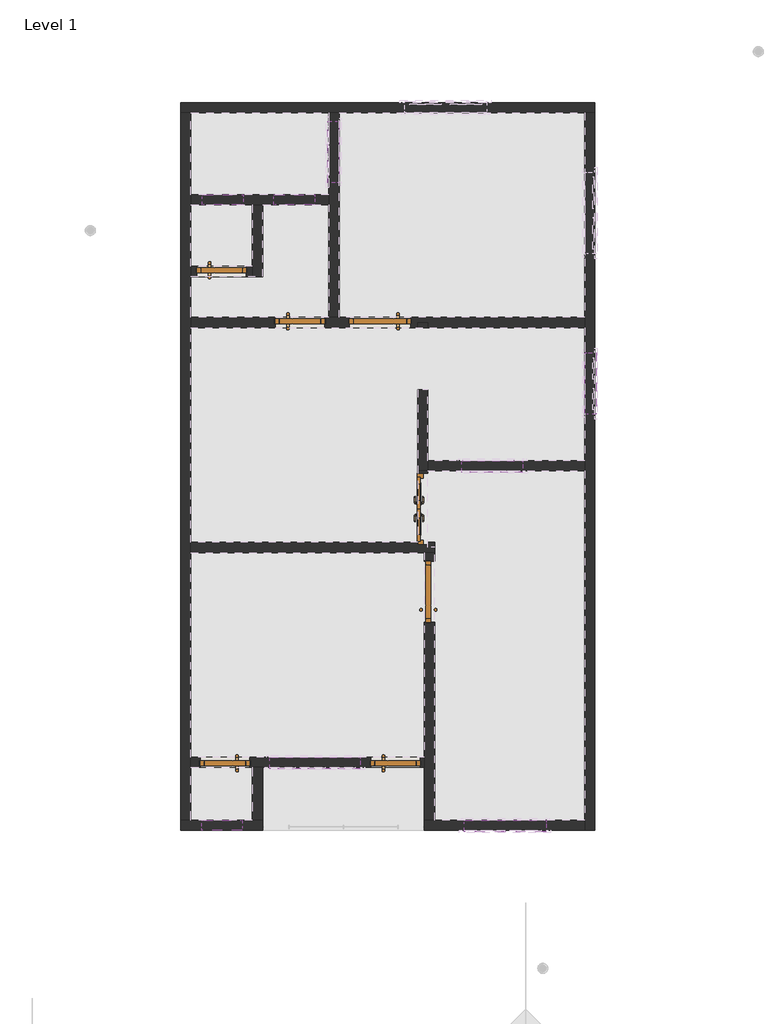
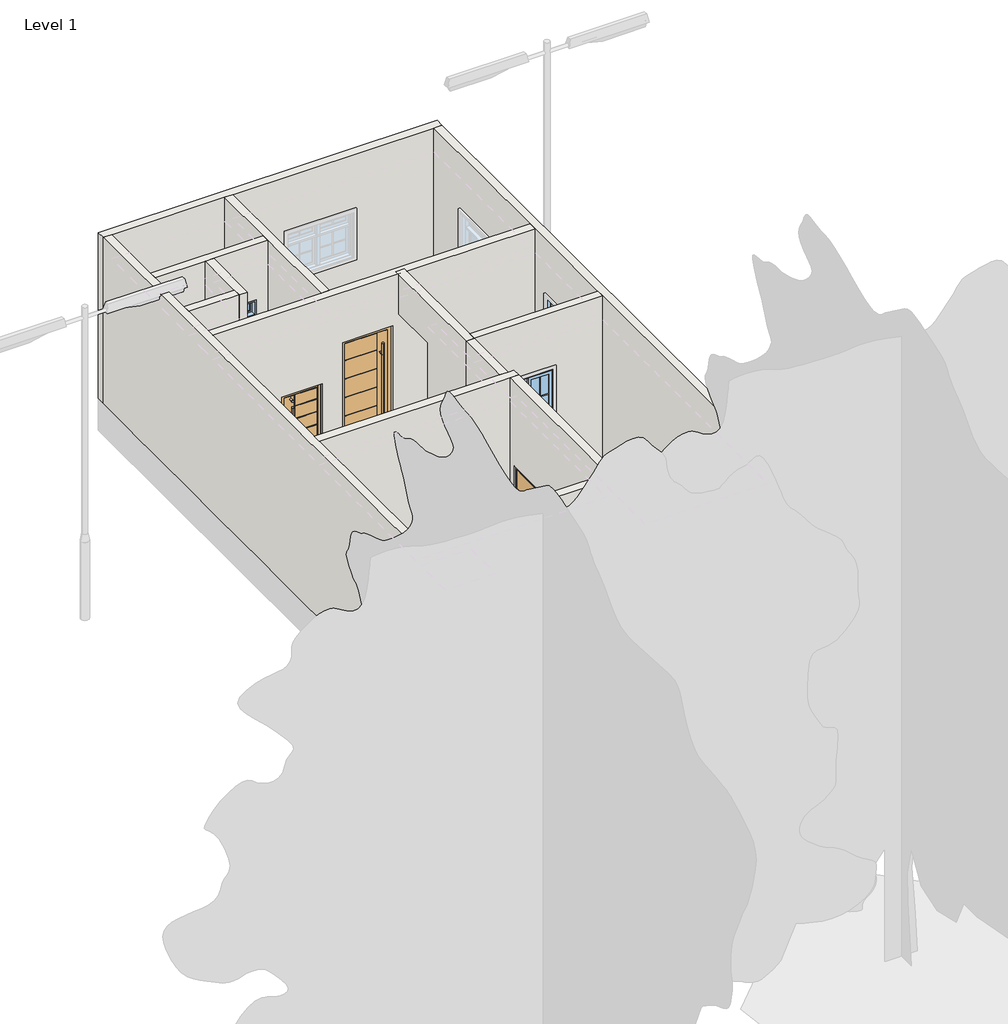
# One storey, part 1 of 2: 17 walls, 8 windows, 7 doors.
"""IFC4 building model written with IfcOpenShell, lengths in millimetres."""

from ifc_helpers import new_model, si_unit, frame, origin, place, context, project, spatial, polyline, outline, extrude, faceted_brep, transform, mapped, element, save
from components import door_9b787682, door_dc81b0c5, door_3_5c4206ef, door_3_79df91aa, door_2576ec39, door_55c03dfd, fixed_2_65c13adb, window_61697a4f, m_window_casement_double_3_e0bd8fa3, m_window_casement_double_awning_double_4_7efa9bbd

model = new_model("IFC4")

# Units and contexts
model_context = context("Model", 3, world=origin())
ifc_project = project(units=[si_unit("LENGTHUNIT", "METRE", prefix="MILLI")], contexts=[model_context])

# Site, building, storey
site = spatial("IfcSite", under=ifc_project)
building = spatial("IfcBuilding", under=site)
storey = spatial("IfcBuildingStorey", under=building, Name="Level 1", Elevation=0.0)

# Doors
placement = place(None, origin())
door_shape = door_9b787682(model_context)
element("IfcDoor", 1, ObjectType="2'5\"", at=placement, inside=storey, context=model_context, shape_type="MappedRepresentation", body=[
    mapped(door_shape, transform((-22033.2963079, 3049.4742053, 655.8445349), x_axis=(1.0, 0.0, 0.0), y_axis=(0.0, 1.0, 0.0), z_axis=(0.0, 0.0, 1.0))),
])
element("IfcDoor", 2, ObjectType="2'5\"", at=placement, inside=storey, context=model_context, shape_type="MappedRepresentation", body=[
    mapped(door_shape, transform((-23201.6963079, 3811.4742053, 655.8445349), x_axis=(1.0, 0.0, 0.0), y_axis=(0.0, 1.0, 0.0), z_axis=(0.0, 0.0, 1.0))),
])
element("IfcDoor", 3, ObjectType="2'5\"", at=placement, inside=storey, context=model_context, shape_type="MappedRepresentation", body=[
    mapped(door_shape, transform((-23150.8963079, -3503.7257947, 655.8445349), x_axis=(-1.0, 0.0, 0.0), y_axis=(0.0, -1.0, 0.0), z_axis=(0.0, 0.0, 1.0))),
])
door_2_shape = door_dc81b0c5(model_context)
element("IfcDoor", 4, ObjectType="2'5\"", at=placement, inside=storey, context=model_context, shape_type="MappedRepresentation", body=[
    mapped(door_2_shape, transform((-20610.8963079, -3503.7257947, 655.8445349), x_axis=(1.0, 0.0, 0.0), y_axis=(0.0, 1.0, 0.0), z_axis=(0.0, 0.0, 1.0))),
])
door_3_shape = door_3_5c4206ef(model_context)
element("IfcDoor", 5, ObjectType="3'", at=placement, inside=storey, context=model_context, shape_type="MappedRepresentation", body=[
    mapped(door_3_shape, transform((-20102.8963079, -963.7257947, 0.0), x_axis=(0.0, 1.0, 0.0), y_axis=(-1.0, 0.0, 0.0), z_axis=(0.0, 0.0, 1.0))),
])
door_3_2_shape = door_3_79df91aa(model_context)
element("IfcDoor", 6, ObjectType="3'", at=placement, inside=storey, context=model_context, shape_type="MappedRepresentation", body=[
    mapped(door_3_2_shape, transform((-20839.4963079, 3049.4742053, 655.8445349), x_axis=(-1.0, 0.0, 0.0), y_axis=(0.0, -1.0, 0.0), z_axis=(0.0, 0.0, 1.0))),
])
door_4_shape = door_2576ec39(model_context)
door_5_shape = door_55c03dfd(model_context)
element("IfcDoor", 7, ObjectType="ExtDbl (8) : 3'6\"", at=placement, inside=storey, context=model_context, shape_type="MappedRepresentation", body=[
    mapped(door_4_shape, transform((-20204.4963079, 268.1742053, 0.0), x_axis=(0.0, -1.0, 0.0), y_axis=(1.0, 0.0, 0.0), z_axis=(0.0, 0.0, 1.0))),
    mapped(door_5_shape, transform((-20204.4963079, 268.1742053, 0.0), x_axis=(0.0, -1.0, 0.0), y_axis=(1.0, 0.0, 0.0), z_axis=(0.0, 0.0, 1.0))),
])

# Walls
element("IfcWall", 8, ObjectType="Generic - 6\"", at=placement, inside=storey, context=model_context, shape_type="Brep", body=[
    faceted_brep([(-23811.2963079, 6173.6742053, 609.6), (-23658.8963079, 6173.6742053, 609.6), (-21601.4963079, 6173.6742053, 609.6), (-21449.0963079, 6173.6742053, 609.6), (-17791.4963079, 6173.6742053, 609.6), (-17639.0963079, 6173.6742053, 609.6), (-17639.0963079, 6173.6742053, 3810.0), (-17791.4963079, 6173.6742053, 3810.0), (-21449.0963079, 6173.6742053, 3810.0), (-21601.4963079, 6173.6742053, 3810.0), (-23658.8963079, 6173.6742053, 3810.0), (-23811.2963079, 6173.6742053, 3810.0), (-19251.9963079, 6173.6742053, 2728.8), (-19251.9963079, 6173.6742053, 1828.8), (-20471.1963079, 6173.6742053, 1828.8), (-20471.1963079, 6173.6742053, 2728.8), (-23811.2963079, 6326.0742053, 609.6), (-23811.2963079, 6326.0742053, 3810.0), (-17639.0963079, 6326.0742053, 3810.0), (-17639.0963079, 6326.0742053, 609.6), (-19251.9963079, 6326.0742053, 2728.8), (-20471.1963079, 6326.0742053, 2728.8), (-20471.1963079, 6326.0742053, 1828.8), (-19251.9963079, 6326.0742053, 1828.8)], [[[0, 1, 2, 3, 4, 5, 6, 7, 8, 9, 10, 11], [12, 13, 14, 15]], [[16, 17, 18, 19], [20, 21, 22, 23]], [[5, 4, 3, 2, 1, 0, 16, 19]], [[11, 10, 9, 8, 7, 6, 18, 17]], [[6, 5, 19, 18]], [[0, 11, 17, 16]], [[13, 12, 20, 23]], [[14, 13, 23, 22]], [[15, 14, 22, 21]], [[12, 15, 21, 20]]]),
])
element("IfcWall", 9, ObjectType="Generic - 6\"", at=placement, inside=storey, context=model_context, shape_type="Brep", body=[
    faceted_brep([(-17791.4963079, 6173.6742053, 609.6), (-17791.4963079, 3125.6742053, 609.6), (-17791.4963079, 2973.2742053, 609.6), (-17791.4963079, 992.0742053, 609.6), (-17791.4963079, 839.6742053, 609.6), (-17791.4963079, -4367.3257947, 609.6), (-17791.4963079, -4519.7257947, 609.6), (-17791.4963079, -4519.7257947, 3810.0), (-17791.4963079, -4367.3257947, 3810.0), (-17791.4963079, 839.6742053, 3810.0), (-17791.4963079, 992.0742053, 3810.0), (-17791.4963079, 2973.2742053, 3810.0), (-17791.4963079, 3125.6742053, 3810.0), (-17791.4963079, 6173.6742053, 3810.0), (-17791.4963079, 4071.8242053, 2728.8), (-17791.4963079, 4071.8242053, 1828.8), (-17791.4963079, 5291.0242053, 1828.8), (-17791.4963079, 5291.0242053, 2728.8), (-17791.4963079, 1682.6367053, 2728.8), (-17791.4963079, 1682.6367053, 1828.8), (-17791.4963079, 2597.0367053, 1828.8), (-17791.4963079, 2597.0367053, 2728.8), (-17639.0963079, 6173.6742053, 609.6), (-17639.0963079, 6173.6742053, 3810.0), (-17639.0963079, -4519.7257947, 3810.0), (-17639.0963079, -4519.7257947, 609.6), (-17639.0963079, 4071.8242053, 2728.8), (-17639.0963079, 5291.0242053, 2728.8), (-17639.0963079, 5291.0242053, 1828.8), (-17639.0963079, 4071.8242053, 1828.8), (-17639.0963079, 1682.6367053, 2728.8), (-17639.0963079, 2597.0367053, 2728.8), (-17639.0963079, 2597.0367053, 1828.8), (-17639.0963079, 1682.6367053, 1828.8)], [[[0, 1, 2, 3, 4, 5, 6, 7, 8, 9, 10, 11, 12, 13], [14, 15, 16, 17], [18, 19, 20, 21]], [[22, 23, 24, 25], [26, 27, 28, 29], [30, 31, 32, 33]], [[6, 5, 4, 3, 2, 1, 0, 22, 25]], [[13, 12, 11, 10, 9, 8, 7, 24, 23]], [[0, 13, 23, 22]], [[7, 6, 25, 24]], [[15, 14, 26, 29]], [[16, 15, 29, 28]], [[17, 16, 28, 27]], [[14, 17, 27, 26]], [[19, 18, 30, 33]], [[20, 19, 33, 32]], [[21, 20, 32, 31]], [[18, 21, 31, 30]]]),
])
element("IfcWall", 10, ObjectType="Generic - 6\"", at=placement, inside=storey, context=model_context, shape_type="Brep", body=[
    faceted_brep([(-17791.4963079, -4367.3257947, 609.6), (-20026.6963079, -4367.3257947, 609.6), (-20179.0963079, -4367.3257947, 609.6), (-20179.0963079, -4367.3257947, 3810.0), (-20026.6963079, -4367.3257947, 3810.0), (-17791.4963079, -4367.3257947, 3810.0), (-19585.5697454, -4367.3257947, 2728.8), (-19585.5697454, -4367.3257947, 1828.8), (-18366.3697454, -4367.3257947, 1828.8), (-18366.3697454, -4367.3257947, 2728.8), (-17791.4963079, -4519.7257947, 609.6), (-17791.4963079, -4519.7257947, 3810.0), (-20179.0963079, -4519.7257947, 3810.0), (-20179.0963079, -4519.7257947, 609.6), (-19585.5697454, -4519.7257947, 2728.8), (-18366.3697454, -4519.7257947, 2728.8), (-18366.3697454, -4519.7257947, 1828.8), (-19585.5697454, -4519.7257947, 1828.8)], [[[0, 1, 2, 3, 4, 5], [6, 7, 8, 9]], [[10, 11, 12, 13], [14, 15, 16, 17]], [[2, 1, 0, 10, 13]], [[5, 4, 3, 12, 11]], [[0, 5, 11, 10]], [[3, 2, 13, 12]], [[7, 6, 14, 17]], [[8, 7, 17, 16]], [[9, 8, 16, 15]], [[6, 9, 15, 14]]]),
])
element("IfcWall", 11, ObjectType="Generic - 6\"", at=placement, inside=storey, context=model_context, shape_type="Brep", body=[
    faceted_brep([(-23811.2963079, -4519.7257947, 609.6), (-22592.0963079, -4519.7257947, 609.6), (-22592.0963079, -4519.7257947, 3810.0), (-23811.2963079, -4519.7257947, 3810.0), (-23500.5431829, -4519.7257947, 2743.2), (-22890.9431829, -4519.7257947, 2743.2), (-22890.9431829, -4519.7257947, 2438.4), (-23500.5431829, -4519.7257947, 2438.4), (-23811.2963079, -4367.3257947, 609.6), (-23811.2963079, -4367.3257947, 3810.0), (-23658.8963079, -4367.3257947, 3810.0), (-22744.4963079, -4367.3257947, 3810.0), (-22592.0963079, -4367.3257947, 3810.0), (-22592.0963079, -4367.3257947, 609.6), (-22744.4963079, -4367.3257947, 609.6), (-23658.8963079, -4367.3257947, 609.6), (-23500.5431829, -4367.3257947, 2743.2), (-23500.5431829, -4367.3257947, 2438.4), (-22890.9431829, -4367.3257947, 2438.4), (-22890.9431829, -4367.3257947, 2743.2)], [[[0, 1, 2, 3], [4, 5, 6, 7]], [[8, 9, 10, 11, 12, 13, 14, 15], [16, 17, 18, 19]], [[1, 0, 8, 15, 14, 13]], [[3, 2, 12, 11, 10, 9]], [[0, 3, 9, 8]], [[2, 1, 13, 12]], [[17, 16, 4, 7]], [[18, 17, 7, 6]], [[19, 18, 6, 5]], [[16, 19, 5, 4]]]),
])
element("IfcWall", 12, ObjectType="Generic - 6\"", at=placement, inside=storey, context=model_context, shape_type="Brep", body=[
    faceted_brep([(-23658.8963079, -4367.3257947, 609.6), (-23658.8963079, -3579.9257947, 609.6), (-23658.8963079, -3427.5257947, 609.6), (-23658.8963079, -379.5257947, 609.6), (-23658.8963079, -227.1257947, 609.6), (-23658.8963079, 2973.2742053, 609.6), (-23658.8963079, 3125.6742053, 609.6), (-23658.8963079, 3735.2742053, 609.6), (-23658.8963079, 3887.6742053, 609.6), (-23658.8963079, 4802.0742053, 609.6), (-23658.8963079, 4954.4742053, 609.6), (-23658.8963079, 6173.6742053, 609.6), (-23658.8963079, 6173.6742053, 3810.0), (-23658.8963079, 4954.4742053, 3810.0), (-23658.8963079, 4802.0742053, 3810.0), (-23658.8963079, 3887.6742053, 3810.0), (-23658.8963079, 3735.2742053, 3810.0), (-23658.8963079, 3125.6742053, 3810.0), (-23658.8963079, 2973.2742053, 3810.0), (-23658.8963079, -227.1257947, 3810.0), (-23658.8963079, -379.5257947, 3810.0), (-23658.8963079, -3427.5257947, 3810.0), (-23658.8963079, -3579.9257947, 3810.0), (-23658.8963079, -4367.3257947, 3810.0), (-23811.2963079, -4367.3257947, 609.6), (-23811.2963079, -4367.3257947, 3810.0), (-23811.2963079, 6173.6742053, 3810.0), (-23811.2963079, 6173.6742053, 609.6)], [[[0, 1, 2, 3, 4, 5, 6, 7, 8, 9, 10, 11, 12, 13, 14, 15, 16, 17, 18, 19, 20, 21, 22, 23]], [[24, 25, 26, 27]], [[11, 10, 9, 8, 7, 6, 5, 4, 3, 2, 1, 0, 24, 27]], [[23, 22, 21, 20, 19, 18, 17, 16, 15, 14, 13, 12, 26, 25]], [[12, 11, 27, 26]], [[0, 23, 25, 24]]]),
])
element("IfcWall", 13, ObjectType="Generic - 6\"", at=placement, inside=storey, context=model_context, shape_type="Brep", body=[
    faceted_brep([(-21601.4963079, 6173.6742053, 609.6), (-21601.4963079, 4954.4742053, 609.6), (-21601.4963079, 4802.0742053, 609.6), (-21601.4963079, 3125.6742053, 609.6), (-21601.4963079, 3125.6742053, 3810.0), (-21601.4963079, 4802.0742053, 3810.0), (-21601.4963079, 4954.4742053, 3810.0), (-21601.4963079, 6173.6742053, 3810.0), (-21601.4963079, 6046.6742053, 2728.8), (-21601.4963079, 5132.2742053, 2728.8), (-21601.4963079, 5132.2742053, 1828.8), (-21601.4963079, 6046.6742053, 1828.8), (-21449.0963079, 6173.6742053, 609.6), (-21449.0963079, 6173.6742053, 3810.0), (-21449.0963079, 3125.6742053, 3810.0), (-21449.0963079, 3125.6742053, 609.6), (-21449.0963079, 6046.6742053, 2728.8), (-21449.0963079, 6046.6742053, 1828.8), (-21449.0963079, 5132.2742053, 1828.8), (-21449.0963079, 5132.2742053, 2728.8)], [[[0, 1, 2, 3, 4, 5, 6, 7], [8, 9, 10, 11]], [[12, 13, 14, 15], [16, 17, 18, 19]], [[3, 2, 1, 0, 12, 15]], [[7, 6, 5, 4, 14, 13]], [[0, 7, 13, 12]], [[4, 3, 15, 14]], [[17, 16, 8, 11]], [[18, 17, 11, 10]], [[19, 18, 10, 9]], [[16, 19, 9, 8]]]),
])
element("IfcWall", 14, ObjectType="Generic - 6\"", at=placement, inside=storey, context=model_context, shape_type="Brep", body=[
    faceted_brep([(-23658.8963079, 2973.2742053, 609.6), (-17791.4963079, 2973.2742053, 609.6), (-17791.4963079, 2973.2742053, 3810.0), (-23658.8963079, 2973.2742053, 3810.0), (-21296.6963079, 2973.2742053, 2845.3445349), (-20382.2963079, 2973.2742053, 2845.3445349), (-20382.2963079, 2973.2742053, 655.8445349), (-21296.6963079, 2973.2742053, 655.8445349), (-22401.5963079, 2973.2742053, 2179.8445349), (-21664.9963079, 2973.2742053, 2179.8445349), (-21664.9963079, 2973.2742053, 655.8445349), (-22401.5963079, 2973.2742053, 655.8445349), (-17791.4963079, 3125.6742053, 609.6), (-21449.0963079, 3125.6742053, 609.6), (-21601.4963079, 3125.6742053, 609.6), (-23658.8963079, 3125.6742053, 609.6), (-23658.8963079, 3125.6742053, 3810.0), (-21601.4963079, 3125.6742053, 3810.0), (-21449.0963079, 3125.6742053, 3810.0), (-17791.4963079, 3125.6742053, 3810.0), (-20382.2963079, 3125.6742053, 2845.3445349), (-21296.6963079, 3125.6742053, 2845.3445349), (-21296.6963079, 3125.6742053, 655.8445349), (-20382.2963079, 3125.6742053, 655.8445349), (-21664.9963079, 3125.6742053, 2179.8445349), (-22401.5963079, 3125.6742053, 2179.8445349), (-22401.5963079, 3125.6742053, 655.8445349), (-21664.9963079, 3125.6742053, 655.8445349), (-21296.6963079, 3105.6742053, 2845.3445349), (-20382.2963079, 3105.6742053, 2845.3445349), (-20382.2963079, 3028.6742053, 2845.3445349), (-21296.6963079, 3028.6742053, 2845.3445349), (-21296.6963079, 3105.6742053, 655.8445349), (-21296.6963079, 3028.6742053, 655.8445349), (-21311.6963079, 3105.6742053, 655.8445349), (-21311.6963079, 3028.6742053, 655.8445349), (-20382.2963079, 3028.6742053, 655.8445349), (-20367.2963079, 3028.6742053, 655.8445349), (-20367.2963079, 3105.6742053, 655.8445349), (-20382.2963079, 3105.6742053, 655.8445349), (-21311.6963079, 3105.6742053, 2860.3445349), (-20367.2963079, 3105.6742053, 2860.3445349), (-20367.2963079, 3028.6742053, 2860.3445349), (-21311.6963079, 3028.6742053, 2860.3445349), (-21664.9963079, 3105.6742053, 2179.8445349), (-22401.5963079, 3105.6742053, 2179.8445349), (-22401.5963079, 3028.6742053, 2179.8445349), (-21664.9963079, 3028.6742053, 2179.8445349), (-21664.9963079, 3105.6742053, 655.8445349), (-21664.9963079, 3028.6742053, 655.8445349), (-22401.5963079, 3105.6742053, 655.8445349), (-22416.5963079, 3105.6742053, 655.8445349), (-22416.5963079, 3028.6742053, 655.8445349), (-22401.5963079, 3028.6742053, 655.8445349), (-21649.9963079, 3028.6742053, 655.8445349), (-21649.9963079, 3105.6742053, 655.8445349), (-22416.5963079, 3105.6742053, 2194.8445349), (-21649.9963079, 3105.6742053, 2194.8445349), (-21649.9963079, 3028.6742053, 2194.8445349), (-22416.5963079, 3028.6742053, 2194.8445349)], [[[0, 1, 2, 3], [4, 5, 6, 7], [8, 9, 10, 11]], [[12, 13, 14, 15, 16, 17, 18, 19], [20, 21, 22, 23], [24, 25, 26, 27]], [[1, 0, 15, 14, 13, 12]], [[3, 2, 19, 18, 17, 16]], [[2, 1, 12, 19]], [[0, 3, 16, 15]], [[28, 21, 20, 29]], [[30, 5, 4, 31]], [[21, 28, 32, 22]], [[31, 4, 7, 33]], [[22, 32, 34, 35, 33, 7, 6, 36, 37, 38, 39, 23]], [[29, 20, 23, 39]], [[5, 30, 36, 6]], [[40, 41, 42, 43]], [[35, 34, 40, 43]], [[30, 31, 33, 35, 43, 42, 37, 36]], [[38, 37, 42, 41]], [[28, 29, 39, 38, 41, 40, 34, 32]], [[24, 44, 45, 25]], [[8, 46, 47, 9]], [[44, 24, 27, 48]], [[9, 47, 49, 10]], [[48, 27, 26, 50, 51, 52, 53, 11, 10, 49, 54, 55]], [[25, 45, 50, 26]], [[46, 8, 11, 53]], [[56, 57, 58, 59]], [[55, 54, 58, 57]], [[47, 46, 53, 52, 59, 58, 54, 49]], [[52, 51, 56, 59]], [[45, 44, 48, 55, 57, 56, 51, 50]]]),
])
element("IfcWall", 15, ObjectType="Generic - 6\"", at=placement, inside=storey, context=model_context, shape_type="Brep", body=[
    faceted_brep([(-20280.6963079, 839.6742053, 609.6), (-20280.6963079, 839.6742053, 3810.0), (-20280.6963079, 3049.4742053, 3810.0), (-20280.6963079, 3049.4742053, 609.6), (-20280.6963079, 2974.7724011, 609.6), (-20280.6963079, 2974.7724011, 3048.0), (-20280.6963079, 2050.5574639, 3048.0), (-20280.6963079, 2050.5574639, 609.6), (-20128.2963079, 839.6742053, 3810.0), (-20128.2963079, 839.6742053, 609.6), (-20128.2963079, 992.0742053, 609.6), (-20128.2963079, 2050.5574639, 609.6), (-20128.2963079, 2050.5574639, 3048.0), (-20128.2963079, 2974.7724011, 3048.0), (-20128.2963079, 2974.7724011, 609.6), (-20128.2963079, 3049.4742053, 609.6), (-20128.2963079, 3049.4742053, 3810.0), (-20128.2963079, 992.0742053, 3810.0)], [[[0, 1, 2, 3, 4, 5, 6, 7]], [[8, 9, 10, 11, 12, 13, 14, 15, 16, 17]], [[3, 15, 14, 4]], [[9, 0, 7, 11, 10]], [[2, 1, 8, 17, 16]], [[3, 2, 16, 15]], [[1, 0, 9, 8]], [[5, 13, 12, 6]], [[13, 5, 4, 14]], [[6, 12, 11, 7]]]),
])
element("IfcWall", 16, ObjectType="Generic - 6\"", at=placement, inside=storey, context=model_context, shape_type="SweptSolid", body=[
    extrude(outline(polyline([(609.6, -20128.2963079), (609.6, -17791.4963079), (3810.0, -17791.4963079), (3810.0, -20128.2963079), (609.6, -20128.2963079)]), holes=[polyline([(2728.8, -19624.1658391), (2728.8, -18709.7658391), (1828.8, -18709.7658391), (1828.8, -19624.1658391), (2728.8, -19624.1658391)])]), frame((0.0, 839.6742053, 0.0), z_axis=(0.0, 1.0, 0.0), x_axis=(0.0, 0.0, 1.0)), (0.0, 0.0, 1.0), 152.4),
])
element("IfcWall", 17, ObjectType="Generic - 6\"", at=placement, inside=storey, context=model_context, shape_type="Brep", body=[
    faceted_brep([(-23658.8963079, -379.5257947, 609.6), (-20179.0963079, -379.5257947, 609.6), (-20026.6963079, -379.5257947, 609.6), (-20026.6963079, -379.5257947, 3810.0), (-20179.0963079, -379.5257947, 3810.0), (-23658.8963079, -379.5257947, 3810.0), (-23658.8963079, -227.1257947, 3810.0), (-20280.6963079, -227.1257947, 3810.0), (-20128.2963079, -227.1257947, 3810.0), (-20026.6963079, -227.1257947, 3810.0), (-20026.6963079, -227.1257947, 609.6), (-20128.2963079, -227.1257947, 609.6), (-20128.2963079, -227.1257947, 2110.0), (-20280.6963079, -227.1257947, 2110.0), (-20280.6963079, -227.1257947, 609.6), (-23658.8963079, -227.1257947, 609.6), (-20280.6963079, -265.2257947, 609.6), (-20128.2963079, -265.2257947, 609.6), (-20280.6963079, -265.2257947, 2110.0), (-20128.2963079, -265.2257947, 2110.0)], [[[0, 1, 2, 3, 4, 5]], [[6, 7, 8, 9, 10, 11, 12, 13, 14, 15]], [[2, 1, 0, 15, 14, 16, 17, 11, 10]], [[5, 4, 3, 9, 8, 7, 6]], [[0, 5, 6, 15]], [[3, 2, 10, 9]], [[13, 18, 16, 14]], [[17, 19, 12, 11]], [[19, 18, 13, 12]], [[18, 19, 17, 16]]]),
])
element("IfcWall", 18, ObjectType="Generic - 6\"", at=placement, inside=storey, context=model_context, shape_type="Brep", body=[
    faceted_brep([(-20179.0963079, -4367.3257947, 3810.0), (-20179.0963079, -3579.9257947, 3810.0), (-20179.0963079, -3427.5257947, 3810.0), (-20179.0963079, -379.5257947, 3810.0), (-20179.0963079, -379.5257947, 609.6), (-20179.0963079, -506.5257947, 609.6), (-20179.0963079, -506.5257947, 2189.5), (-20179.0963079, -1420.9257947, 2189.5), (-20179.0963079, -1420.9257947, 609.6), (-20179.0963079, -3427.5257947, 609.6), (-20179.0963079, -3579.9257947, 609.6), (-20179.0963079, -4367.3257947, 609.6), (-20026.6963079, -379.5257947, 3810.0), (-20026.6963079, -4367.3257947, 3810.0), (-20026.6963079, -4367.3257947, 609.6), (-20026.6963079, -1420.9257947, 609.6), (-20026.6963079, -1420.9257947, 2189.5), (-20026.6963079, -506.5257947, 2189.5), (-20026.6963079, -506.5257947, 609.6), (-20026.6963079, -379.5257947, 609.6), (-20082.0963079, -506.5257947, 609.6), (-20082.0963079, -491.5257947, 609.6), (-20159.0963079, -491.5257947, 609.6), (-20159.0963079, -506.5257947, 609.6), (-20159.0963079, -1420.9257947, 609.6), (-20159.0963079, -1435.9257947, 609.6), (-20082.0963079, -1435.9257947, 609.6), (-20082.0963079, -1420.9257947, 609.6), (-20159.0963079, -506.5257947, 2189.5), (-20159.0963079, -1420.9257947, 2189.5), (-20082.0963079, -1420.9257947, 2189.5), (-20082.0963079, -506.5257947, 2189.5), (-20159.0963079, -1435.9257947, 2204.5), (-20159.0963079, -491.5257947, 2204.5), (-20082.0963079, -491.5257947, 2204.5), (-20082.0963079, -1435.9257947, 2204.5)], [[[0, 1, 2, 3, 4, 5, 6, 7, 8, 9, 10, 11]], [[12, 13, 14, 15, 16, 17, 18, 19]], [[4, 19, 18, 20, 21, 22, 23, 5]], [[14, 11, 10, 9, 8, 24, 25, 26, 27, 15]], [[3, 2, 1, 0, 13, 12]], [[0, 11, 14, 13]], [[4, 3, 12, 19]], [[6, 28, 29, 7]], [[16, 30, 31, 17]], [[28, 6, 5, 23]], [[17, 31, 20, 18]], [[7, 29, 24, 8]], [[30, 16, 15, 27]], [[32, 33, 34, 35]], [[34, 33, 22, 21]], [[31, 30, 27, 26, 35, 34, 21, 20]], [[32, 35, 26, 25]], [[29, 28, 23, 22, 33, 32, 25, 24]]]),
])
element("IfcWall", 19, ObjectType="Generic - 6\"", at=placement, inside=storey, context=model_context, shape_type="Brep", body=[
    faceted_brep([(-23658.8963079, -3579.9257947, 609.6), (-22744.4963079, -3579.9257947, 609.6), (-22592.0963079, -3579.9257947, 609.6), (-20179.0963079, -3579.9257947, 609.6), (-20179.0963079, -3579.9257947, 3810.0), (-22592.0963079, -3579.9257947, 3810.0), (-22744.4963079, -3579.9257947, 3810.0), (-23658.8963079, -3579.9257947, 3810.0), (-22484.1463079, -3579.9257947, 1828.8), (-22484.1463079, -3579.9257947, 2628.8), (-21137.9463079, -3579.9257947, 2628.8), (-21137.9463079, -3579.9257947, 1828.8), (-20979.1963079, -3579.9257947, 2179.8445349), (-20242.5963079, -3579.9257947, 2179.8445349), (-20242.5963079, -3579.9257947, 655.8445349), (-20979.1963079, -3579.9257947, 655.8445349), (-23519.1963079, -3579.9257947, 2179.8445349), (-22782.5963079, -3579.9257947, 2179.8445349), (-22782.5963079, -3579.9257947, 655.8445349), (-23519.1963079, -3579.9257947, 655.8445349), (-20179.0963079, -3427.5257947, 609.6), (-23658.8963079, -3427.5257947, 609.6), (-23658.8963079, -3427.5257947, 3810.0), (-20179.0963079, -3427.5257947, 3810.0), (-22484.1463079, -3427.5257947, 2628.8), (-22484.1463079, -3427.5257947, 1828.8), (-21137.9463079, -3427.5257947, 1828.8), (-21137.9463079, -3427.5257947, 2628.8), (-20242.5963079, -3427.5257947, 2179.8445349), (-20979.1963079, -3427.5257947, 2179.8445349), (-20979.1963079, -3427.5257947, 655.8445349), (-20242.5963079, -3427.5257947, 655.8445349), (-22782.5963079, -3427.5257947, 2179.8445349), (-23519.1963079, -3427.5257947, 2179.8445349), (-23519.1963079, -3427.5257947, 655.8445349), (-22782.5963079, -3427.5257947, 655.8445349), (-20979.1963079, -3559.9257947, 2179.8445349), (-20242.5963079, -3559.9257947, 2179.8445349), (-20242.5963079, -3482.9257947, 2179.8445349), (-20979.1963079, -3482.9257947, 2179.8445349), (-20242.5963079, -3559.9257947, 655.8445349), (-20242.5963079, -3482.9257947, 655.8445349), (-20227.5963079, -3559.9257947, 655.8445349), (-20227.5963079, -3482.9257947, 655.8445349), (-20979.1963079, -3482.9257947, 655.8445349), (-20994.1963079, -3482.9257947, 655.8445349), (-20994.1963079, -3559.9257947, 655.8445349), (-20979.1963079, -3559.9257947, 655.8445349), (-20994.1963079, -3559.9257947, 2194.8445349), (-20994.1963079, -3482.9257947, 2194.8445349), (-20227.5963079, -3482.9257947, 2194.8445349), (-20227.5963079, -3559.9257947, 2194.8445349), (-23519.1963079, -3559.9257947, 2179.8445349), (-22782.5963079, -3559.9257947, 2179.8445349), (-22782.5963079, -3482.9257947, 2179.8445349), (-23519.1963079, -3482.9257947, 2179.8445349), (-23519.1963079, -3559.9257947, 655.8445349), (-23519.1963079, -3482.9257947, 655.8445349), (-22782.5963079, -3559.9257947, 655.8445349), (-22767.5963079, -3559.9257947, 655.8445349), (-22767.5963079, -3482.9257947, 655.8445349), (-22782.5963079, -3482.9257947, 655.8445349), (-23534.1963079, -3482.9257947, 655.8445349), (-23534.1963079, -3559.9257947, 655.8445349), (-22767.5963079, -3559.9257947, 2194.8445349), (-23534.1963079, -3559.9257947, 2194.8445349), (-23534.1963079, -3482.9257947, 2194.8445349), (-22767.5963079, -3482.9257947, 2194.8445349)], [[[0, 1, 2, 3, 4, 5, 6, 7], [8, 9, 10, 11], [12, 13, 14, 15], [16, 17, 18, 19]], [[20, 21, 22, 23], [24, 25, 26, 27], [28, 29, 30, 31], [32, 33, 34, 35]], [[3, 2, 1, 0, 21, 20]], [[7, 6, 5, 4, 23, 22]], [[0, 7, 22, 21]], [[4, 3, 20, 23]], [[25, 24, 9, 8]], [[26, 25, 8, 11]], [[27, 26, 11, 10]], [[24, 27, 10, 9]], [[12, 36, 37, 13]], [[28, 38, 39, 29]], [[13, 37, 40, 14]], [[38, 28, 31, 41]], [[14, 40, 42, 43, 41, 31, 30, 44, 45, 46, 47, 15]], [[36, 12, 15, 47]], [[29, 39, 44, 30]], [[48, 49, 50, 51]], [[43, 42, 51, 50]], [[39, 38, 41, 43, 50, 49, 45, 44]], [[46, 45, 49, 48]], [[37, 36, 47, 46, 48, 51, 42, 40]], [[16, 52, 53, 17]], [[32, 54, 55, 33]], [[52, 16, 19, 56]], [[33, 55, 57, 34]], [[56, 19, 18, 58, 59, 60, 61, 35, 34, 57, 62, 63]], [[17, 53, 58, 18]], [[54, 32, 35, 61]], [[64, 65, 66, 67]], [[63, 62, 66, 65]], [[55, 54, 61, 60, 67, 66, 62, 57]], [[60, 59, 64, 67]], [[53, 52, 56, 63, 65, 64, 59, 58]]]),
])
element("IfcWall", 20, ObjectType="Generic - 6\"", at=placement, inside=storey, context=model_context, shape_type="SweptSolid", body=[
    extrude(outline(polyline([(-22744.4963079, -4367.3257947), (-22744.4963079, -3579.9257947), (-22592.0963079, -3579.9257947), (-22592.0963079, -4367.3257947), (-22744.4963079, -4367.3257947)])), frame((0.0, 0.0, 609.6), z_axis=(0.0, 0.0, 1.0), x_axis=(1.0, 0.0, 0.0)), (0.0, 0.0, 1.0), 3200.4),
])
element("IfcWall", 21, ObjectType="Generic - 6\"", at=placement, inside=storey, context=model_context, shape_type="Brep", body=[
    faceted_brep([(-23658.8963079, 4802.0742053, 609.6), (-22744.4963079, 4802.0742053, 609.6), (-22592.0963079, 4802.0742053, 609.6), (-21601.4963079, 4802.0742053, 609.6), (-21601.4963079, 4802.0742053, 3810.0), (-22592.0963079, 4802.0742053, 3810.0), (-22744.4963079, 4802.0742053, 3810.0), (-23658.8963079, 4802.0742053, 3810.0), (-22880.5252141, 4802.0742053, 2743.2), (-22880.5252141, 4802.0742053, 2438.4), (-23490.1252141, 4802.0742053, 2438.4), (-23490.1252141, 4802.0742053, 2743.2), (-21812.6338079, 4802.0742053, 2743.2), (-21812.6338079, 4802.0742053, 2438.4), (-22422.2338079, 4802.0742053, 2438.4), (-22422.2338079, 4802.0742053, 2743.2), (-23658.8963079, 4954.4742053, 609.6), (-23658.8963079, 4954.4742053, 3810.0), (-21601.4963079, 4954.4742053, 3810.0), (-21601.4963079, 4954.4742053, 609.6), (-22880.5252141, 4954.4742053, 2743.2), (-23490.1252141, 4954.4742053, 2743.2), (-23490.1252141, 4954.4742053, 2438.4), (-22880.5252141, 4954.4742053, 2438.4), (-21812.6338079, 4954.4742053, 2743.2), (-22422.2338079, 4954.4742053, 2743.2), (-22422.2338079, 4954.4742053, 2438.4), (-21812.6338079, 4954.4742053, 2438.4)], [[[0, 1, 2, 3, 4, 5, 6, 7], [8, 9, 10, 11], [12, 13, 14, 15]], [[16, 17, 18, 19], [20, 21, 22, 23], [24, 25, 26, 27]], [[3, 2, 1, 0, 16, 19]], [[7, 6, 5, 4, 18, 17]], [[0, 7, 17, 16]], [[4, 3, 19, 18]], [[9, 8, 20, 23]], [[10, 9, 23, 22]], [[11, 10, 22, 21]], [[8, 11, 21, 20]], [[13, 12, 24, 27]], [[14, 13, 27, 26]], [[15, 14, 26, 25]], [[12, 15, 25, 24]]]),
])
element("IfcWall", 22, ObjectType="Generic - 6\"", at=placement, inside=storey, context=model_context, shape_type="Brep", body=[
    faceted_brep([(-22744.4963079, 4802.0742053, 609.6), (-22744.4963079, 3887.6742053, 609.6), (-22744.4963079, 3735.2742053, 609.6), (-22744.4963079, 3735.2742053, 3810.0), (-22744.4963079, 3887.6742053, 3810.0), (-22744.4963079, 4802.0742053, 3810.0), (-22592.0963079, 4802.0742053, 609.6), (-22592.0963079, 4802.0742053, 3810.0), (-22592.0963079, 3735.2742053, 3810.0), (-22592.0963079, 3735.2742053, 609.6)], [[[0, 1, 2, 3, 4, 5]], [[6, 7, 8, 9]], [[2, 1, 0, 6, 9]], [[5, 4, 3, 8, 7]], [[0, 5, 7, 6]], [[3, 2, 9, 8]]]),
])
element("IfcWall", 23, ObjectType="Generic - 6\"", at=placement, inside=storey, context=model_context, shape_type="Brep", body=[
    faceted_brep([(-23658.8963079, 3735.2742053, 609.6), (-22744.4963079, 3735.2742053, 609.6), (-22744.4963079, 3735.2742053, 3810.0), (-23658.8963079, 3735.2742053, 3810.0), (-23569.9963079, 3735.2742053, 2179.8445349), (-22833.3963079, 3735.2742053, 2179.8445349), (-22833.3963079, 3735.2742053, 655.8445349), (-23569.9963079, 3735.2742053, 655.8445349), (-22744.4963079, 3887.6742053, 609.6), (-23658.8963079, 3887.6742053, 609.6), (-23658.8963079, 3887.6742053, 3810.0), (-22744.4963079, 3887.6742053, 3810.0), (-22833.3963079, 3887.6742053, 2179.8445349), (-23569.9963079, 3887.6742053, 2179.8445349), (-23569.9963079, 3887.6742053, 655.8445349), (-22833.3963079, 3887.6742053, 655.8445349), (-22833.3963079, 3867.6742053, 2179.8445349), (-23569.9963079, 3867.6742053, 2179.8445349), (-23569.9963079, 3790.6742053, 2179.8445349), (-22833.3963079, 3790.6742053, 2179.8445349), (-22833.3963079, 3867.6742053, 655.8445349), (-22833.3963079, 3790.6742053, 655.8445349), (-23569.9963079, 3867.6742053, 655.8445349), (-23584.9963079, 3867.6742053, 655.8445349), (-23584.9963079, 3790.6742053, 655.8445349), (-23569.9963079, 3790.6742053, 655.8445349), (-22818.3963079, 3790.6742053, 655.8445349), (-22818.3963079, 3867.6742053, 655.8445349), (-23584.9963079, 3867.6742053, 2194.8445349), (-22818.3963079, 3867.6742053, 2194.8445349), (-22818.3963079, 3790.6742053, 2194.8445349), (-23584.9963079, 3790.6742053, 2194.8445349)], [[[0, 1, 2, 3], [4, 5, 6, 7]], [[8, 9, 10, 11], [12, 13, 14, 15]], [[1, 0, 9, 8]], [[3, 2, 11, 10]], [[2, 1, 8, 11]], [[0, 3, 10, 9]], [[12, 16, 17, 13]], [[4, 18, 19, 5]], [[16, 12, 15, 20]], [[5, 19, 21, 6]], [[20, 15, 14, 22, 23, 24, 25, 7, 6, 21, 26, 27]], [[13, 17, 22, 14]], [[18, 4, 7, 25]], [[28, 29, 30, 31]], [[27, 26, 30, 29]], [[19, 18, 25, 24, 31, 30, 26, 21]], [[24, 23, 28, 31]], [[17, 16, 20, 27, 29, 28, 23, 22]]]),
])
element("IfcWall", 24, ObjectType="Generic - 6\"", at=placement, inside=storey, context=model_context, shape_type="SweptSolid", body=[
    extrude(outline(polyline([(-227.1257947, 3810.0), (839.6742053, 3810.0), (839.6742053, 609.6), (801.5742053, 609.6), (801.5742053, 2110.0), (-227.1257947, 2110.0), (-227.1257947, 3810.0)])), frame((-20280.6963079, 0.0, 0.0), z_axis=(1.0, 0.0, 0.0), x_axis=(0.0, 1.0, 0.0)), (0.0, 0.0, 1.0), 152.4),
])

# Windows
fixed_2_shape = fixed_2_65c13adb(model_context)
element("IfcWindow", 25, ObjectType="Fixed : 2'", at=placement, inside=storey, context=model_context, shape_type="MappedRepresentation", body=[
    mapped(fixed_2_shape, transform((-23233.8431829, -4443.5257947, 1524.0), x_axis=(-1.0, 0.0, 0.0), y_axis=(0.0, -1.0, 0.0), z_axis=(0.0, 0.0, 1.0))),
])
element("IfcWindow", 26, ObjectType="Fixed : 2'", at=placement, inside=storey, context=model_context, shape_type="MappedRepresentation", body=[
    mapped(fixed_2_shape, transform((-23147.2252141, 4878.2742053, 1524.0), x_axis=(1.0, 0.0, 0.0), y_axis=(0.0, 1.0, 0.0), z_axis=(0.0, 0.0, 1.0))),
])
element("IfcWindow", 27, ObjectType="Fixed : 2'", at=placement, inside=storey, context=model_context, shape_type="MappedRepresentation", body=[
    mapped(fixed_2_shape, transform((-22079.3338079, 4878.2742053, 1524.0), x_axis=(1.0, 0.0, 0.0), y_axis=(0.0, 1.0, 0.0), z_axis=(0.0, 0.0, 1.0))),
])
window_shape = window_61697a4f(model_context)
element("IfcWindow", 28, ObjectType="M_Window-Awning-Triple-Horizontal : 4'5\"", at=placement, inside=storey, context=model_context, shape_type="MappedRepresentation", body=[
    mapped(window_shape, transform((-21811.0463079, -3503.7257947, 928.8), x_axis=(-1.0, 0.0, 0.0), y_axis=(0.0, -1.0, 0.0), z_axis=(0.0, 0.0, 1.0))),
])
m_window_casement_double_3_shape = m_window_casement_double_3_e0bd8fa3(model_context)
element("IfcWindow", 29, ObjectType="M_Window-Casement-Double : 3'", at=placement, inside=storey, context=model_context, shape_type="MappedRepresentation", body=[
    mapped(m_window_casement_double_3_shape, transform((-19166.9658391, 915.8742053, 928.8), x_axis=(-1.0, 0.0, 0.0), y_axis=(0.0, -1.0, 0.0), z_axis=(0.0, 0.0, 1.0))),
])
element("IfcWindow", 30, ObjectType="M_Window-Casement-Double : 3'", at=placement, inside=storey, context=model_context, shape_type="MappedRepresentation", body=[
    mapped(m_window_casement_double_3_shape, transform((-17715.2963079, 2139.8367053, 928.8), x_axis=(0.0, -1.0, 0.0), y_axis=(1.0, 0.0, 0.0), z_axis=(0.0, 0.0, 1.0))),
])
element("IfcWindow", 31, ObjectType="M_Window-Casement-Double : 3'", at=placement, inside=storey, context=model_context, shape_type="MappedRepresentation", body=[
    mapped(m_window_casement_double_3_shape, transform((-21525.2963079, 5589.4742053, 928.8), x_axis=(0.0, 1.0, 0.0), y_axis=(-1.0, 0.0, 0.0), z_axis=(0.0, 0.0, 1.0))),
])
m_window_casement_double_awning_double_4_shape = m_window_casement_double_awning_double_4_7efa9bbd(model_context)
element("IfcWindow", 32, ObjectType="M_Window-Casement-Double-Awning-Double : 4'", at=placement, inside=storey, context=model_context, shape_type="MappedRepresentation", body=[
    mapped(m_window_casement_double_awning_double_4_shape, transform((-18975.9697454, -4443.5257947, 928.8), x_axis=(-1.0, 0.0, 0.0), y_axis=(0.0, -1.0, 0.0), z_axis=(0.0, 0.0, 1.0))),
])

save(model, "model.ifc")

# Revit data of these elements
# Type "2'5\""
#   Type Mark = "9"
#   Water resistance = "up to Class E900, EN 12208:2001"
#   Uniclass2015Version = "v1.21"
#   Uniclass2015Reference = "Ss_25_30_20_30"
#   Uniclass2015Description = "Frame and door leaf system"
#   URL = "www.aluprof.com"
#   Type IFC Predefined Type = "USERDEFINED"
#   Right-hand / Left-hand door [instance default] = ""
#   Resistance to wind load = "up to Class C5/B5, EN 12210:2001"
#   Insert type = "ST"
#   Hardware [instance default] = ""
#   Product page = "https://aluprof.com/en/architects/offer/window-and-door-systems/panel-doors#visualisation"
#   Operation = "SinglePanelOutwardOpening"
#   Opening type = "Outward"
#   NBSReference = "25-50-20/125"
#   NBSDescription = "Frame and door leaf system"
#   Important = "The actual acceptable construction dimensions are dependent on the selection of profiles and hardware, glazing type, construction weight and the construction’s operating conditions. These should be determined by a suitably qualified person, and using ALUPROF’s calculation software"
#   IfcExportType = "USERDEFINED"
#   IfcExportAs = "IfcDoorType"
#   Handle type [instance default] = ""
#   Manufacturer = "ALUPROF SA"
#   Export Type to IFC As = "IfcDoorType"
#   Door sill type [instance default] = ""
#   Description = "External single-leaf panel door outward opening"
#   Model = "MB-86 ST Panel Door AD07"
#   Content of the recyclate in the material = "69.2%"
#   COBie.Type.WarrantyDurationParts = ""
#   COBie.Type.Name = ""
#   COBie.Type.Manufacturer = "ALUPROF SA"
#   COBie.Space.Name = ""
#   COBie.Floor.Name = ""
#   COBie.Facility.Name = ""
#   COBie.CreatedOn = ""
#   COBie.Component.WarrantyStartDate = ""
#   COBie.Component.Name = "MB-86 ST Panel Door AD07"
#   Burglar resistance = "RC2"
#   Air permeability = "up to Class 4, EN 12207:2001"
#   Width of the active leaf = 2' - 1.17717"
#   Placement in wall = 0' - 0.7874"
#   Thickness = 0' - 3.0315"
#   Height of the opening sash = 4' - 9.44094"
#   Handle Offset = 3' - 5.33858"
#   Rough Height = 5' - 2.40945"
#   Rough Width = 2' - 6.1811"
#   Height = 5' - 0"
#   Width = 2' - 5"
#   Construction depth = 0' - 3.0315"
#   Clear opening width = 1' - 8.94882"
#   Clear opening height = 4' - 8.47638"
#   Height of the array = 0' - 9.08136"
#   Schedule No. [instance default] = 1
#   Handrail [instance default] = yes
#   IsExternal = yes
#   Handle [instance default] = no
#   Door closer [instance default] = no
#   Function = 1
#   COBie.Type = yes
#   COBie = yes
#   Access control [instance default] = no
#   Panel = element 346771
#   Wall Closure = (empty or 0)
# Type "3'"
#   Type Mark = "10"
#   Water resistance = "up to Class E900, EN 12208:2001"
#   Uniclass2015Version = "v1.21"
#   Uniclass2015Reference = "Ss_25_30_20_30"
#   Uniclass2015Description = "Frame and door leaf system"
#   URL = "www.aluprof.com"
#   Type IFC Predefined Type = "USERDEFINED"
#   Right-hand / Left-hand door [instance default] = ""
#   Resistance to wind load = "up to Class C5/B5, EN 12210:2001"
#   Insert type = "ST"
#   Hardware [instance default] = ""
#   Product page = "https://aluprof.com/en/architects/offer/window-and-door-systems/panel-doors#visualisation"
#   Operation = "SinglePanelOutwardOpening"
#   Opening type = "Outward"
#   NBSReference = "25-50-20/125"
#   NBSDescription = "Frame and door leaf system"
#   Important = "The actual acceptable construction dimensions are dependent on the selection of profiles and hardware, glazing type, construction weight and the construction’s operating conditions. These should be determined by a suitably qualified person, and using ALUPROF’s calculation software"
#   IfcExportType = "USERDEFINED"
#   IfcExportAs = "IfcDoorType"
#   Handle type [instance default] = ""
#   Manufacturer = "ALUPROF SA"
#   Export Type to IFC As = "IfcDoorType"
#   Door sill type [instance default] = ""
#   Description = "External single-leaf panel door outward opening"
#   Model = "MB-86 ST Panel Door AD07"
#   Content of the recyclate in the material = "69.2%"
#   COBie.Type.WarrantyDurationParts = ""
#   COBie.Type.Name = ""
#   COBie.Type.Manufacturer = "ALUPROF SA"
#   COBie.Space.Name = ""
#   COBie.Floor.Name = ""
#   COBie.Facility.Name = ""
#   COBie.CreatedOn = ""
#   COBie.Component.WarrantyStartDate = ""
#   COBie.Component.Name = "MB-86 ST Panel Door AD07"
#   Burglar resistance = "RC2"
#   Air permeability = "up to Class 4, EN 12207:2001"
#   Width of the active leaf = 2' - 8.17717"
#   Placement in wall = 0' - 0.7874"
#   Thickness = 0' - 3.0315"
#   Height of the opening sash = 6' - 11.64173"
#   Handle Offset = 3' - 5.33858"
#   Rough Height = 7' - 4.61024"
#   Rough Width = 3' - 1.1811"
#   Height = 7' - 2.20079"
#   Width = 3' - 0"
#   Construction depth = 0' - 3.0315"
#   Clear opening width = 2' - 3.94882"
#   Clear opening height = 6' - 10.67717"
#   Height of the array = 1' - 1.44816"
#   Schedule No. [instance default] = 1
#   Handrail [instance default] = yes
#   IsExternal = yes
#   Handle [instance default] = no
#   Door closer [instance default] = no
#   Function = 1
#   COBie.Type = yes
#   COBie = yes
#   Access control [instance default] = no
#   Panel = element 346771
#   Wall Closure = (empty or 0)
# Type "ExtDbl (8) : 3'6\""
#   Type Mark = "14"
#   Operation = "DoubleDoorSingleSwing"
#   Keynote = "L20"
#   Wrap Layers (Int) from Ext = 0' - 6.98819"
#   Wrap Layers (Ext) from Ext = 0' - 4.03543"
#   Top of Lock Rail = 2' - 11.43307"
#   Thickness = 0' - 1.73228"
#   Stile Shutting = 0' - 4.92126"
#   Stile - Top Rail = 0' - 5.90551"
#   Stile - Lock Rail = 0' - 5.90551"
#   Stile - Hanging = 0' - 3.93701"
#   Stile - Bottom Rail = 0' - 11.81102"
#   Rough Width = 3' - 6"
#   Rough Height = 6' - 11.07087"
#   O/A Frame Width = 0' - 2.51969"
#   Handle Z Distance = 3' - 1.40157"
#   Glazing Thickness = 0' - 0.94488"
#   FrameWidth = 0' - 1.65354"
#   FrameOffset - External = 0' - 2.55906"
#   FrameDepth = 0' - 3.50394"
#   Door Panel Width = 1' - 6.91339"
#   Door Panel Thickness = 0' - 1.73228"
#   Door Panel Height = 6' - 6.74016"
#   Cill Thickness = 0' - 2.14567"
#   Cill Projection = 0' - 1.1811"
#   Handle X Distance = 0' - 2.95276"
#   Height = 6' - 11.07087"
#   Structural Tolerance = 0' - 0.25591"
#   Tolerance = 0' - 0.11811"
#   Undercut = 0' - 0.15748"
#   Width = 3' - 6"
#   Cill Extension = 0' - 0.98425"
#   Cavity Closer Width = 0' - 1.9685"
#   Cavity Closer Offset from Ext = 0' - 4.03543"
#   Cavity Closer Depth = 0' - 3.34646"
#   Vis - Ironmongery = yes
#   Vis - Cavity Closers = yes
#   Function = 1
#   Material Glass = Door - Glazing
#   Handle Style = element 349788
#   Material Door = Door - Panel
#   Material Ironmongery = Door - Handle
#   Wall Closure = (empty or 0)
# Type "Generic - 6\""
#   Assembly Code = "B2010"
#   Layers, outside or top first: 0' - 6" no material (function 1)
# Type "Fixed : 2'"
#   Type Mark = "16"
#   Assembly Code = "B2020100"
#   Height = 1' - 0"
#   Default Sill Height = 3' - 0"
#   Width = 2' - 0"
#   Window Inset = 0' - 0 3/4"
#   Glass Pane Material = Glass
#   Sash Material = Sash
#   Wall Closure = (empty or 0)
# Type "M_Window-Awning-Triple-Horizontal : 4'5\""
#   Type Mark = "15"
#   Fire Rating = "0.5h"
#   Assembly Code = "B2020100"
#   Analytic Construction = "Double glazing - domestic"
#   Window Inset [instance default] = 0' - 0"
#   Wall Thickness [instance default] = 0' - 5.90551"
#   Muntin Width = 1' - 0.33333"
#   Visual Light Transmittance = 0.81
#   Thermal Resistance (R) = 1.8146 (h·ft²·°F)/BTU
#   Solar Heat Gain Coefficient = 0.76
#   One Third Width = 1' - 5.66667"
#   Sash Width = 1' - 4.83333"
#   Rough Width = 4' - 5.59055"
#   Rough Height = 2' - 8.08661"
#   Interior Wall Closure [instance default] = 0' - 2.15551"
#   Height = 2' - 7.49606"
#   Heat Transfer Coefficient (U) = 0.5511 BTU/(h·ft²·°F)
#   Muntin Height = 2' - 1.99606"
#   Frame Extension [instance default] = 0' - 0 1/4"
#   Exterior Wall Closure [instance default] = 0' - 1 1/4"
#   Extension Jamb [instance default] = 0' - 2.15551"
#   Default Sill Height = 2' - 11.43307"
#   Width = 4' - 5"
#   Middle Muntin Visibility = yes
#   Side Muntin Visibility = yes
#   Interior Trim Visibility [instance default] = yes
#   Exterior Trim Visibility [instance default] = yes
#   Extension Jamb Visibility [instance default] = yes
#   Muntin Pattern = M_Muntin Pattern_2x2 : M_Muntin Pattern_2x2
#   Interior Trim Material = Wood - Stained
#   Interior Trim = M_Trim-Window-Interior-Flat : Picture Frame
#   Interior Frame Material = Wood - Stained
#   Glass Panel Material = Glass
#   Exterior Trim Material = Clad - White
#   Exterior Trim = M_Trim-Window-Exterior-Flat : with Sill
#   Exterior Frame Material = Clad - White
#   Wall Closure = (empty or 0)
# Type "M_Window-Casement-Double : 3'"
#   Type Mark = "13"
#   Fire Rating = "0.5h"
#   Assembly Code = "B2020100"
#   Analytic Construction = "Double glazing - domestic"
#   Frame Extension [instance default] = 0' - 0 1/4"
#   Window Inset [instance default] = 0' - 0"
#   Wall Thickness [instance default] = 0' - 5.90551"
#   Interior Wall Closure [instance default] = 0' - 2.15551"
#   Half Width = 1' - 6"
#   Visual Light Transmittance = 0.81
#   Thermal Resistance (R) = 1.8146 (h·ft²·°F)/BTU
#   Solar Heat Gain Coefficient = 0.76
#   Rough Width = 3' - 0.59055"
#   Rough Height = 3' - 0.02362"
#   Height = 2' - 11.43307"
#   Heat Transfer Coefficient (U) = 0.5511 BTU/(h·ft²·°F)
#   Exterior Wall Closure [instance default] = 0' - 1.25197"
#   Extension Jamb [instance default] = 0' - 2.15551"
#   Default Sill Height = 2' - 11.43307"
#   Width = 3' - 0"
#   Muntin Visibility = yes
#   Interior Trim Visibility [instance default] = yes
#   Exterior Trim Visibility [instance default] = yes
#   Extension Jamb Visibility [instance default] = yes
#   Interior Trim Material = Wood - Stained
#   Muntin Pattern = M_Muntin Pattern_2x2 : M_Muntin Pattern_2x2
#   Interior Trim = M_Trim-Window-Interior-Flat : Picture Frame
#   Interior Frame Material = Wood - Stained
#   Glass Panel Material = Glass
#   Exterior Trim Material = Clad - White
#   Exterior Trim = M_Trim-Window-Exterior-Flat : with Sill
#   Exterior Frame Material = Clad - White
#   Wall Closure = (empty or 0)
# Type "M_Window-Casement-Double-Awning-Double : 4'"
#   Type Mark = "11"
#   Fire Rating = "0.5h"
#   Assembly Code = "B2020100"
#   Analytic Construction = "Double glazing - domestic"
#   Window Inset [instance default] = 0' - 0"
#   Wall Thickness [instance default] = 0' - 5.90551"
#   Interior Wall Closure [instance default] = 0' - 2.15551"
#   Half Width = 2' - 0"
#   Visual Light Transmittance = 0.81
#   Transom Height = 0' - 11.81102"
#   Thermal Resistance (R) = 1.8146 (h·ft²·°F)/BTU
#   Solar Heat Gain Coefficient = 0.76
#   Rough Width = 4' - 0.59055"
#   Rough Height = 3' - 0.02362"
#   Open Window Height = 1' - 11.62205"
#   Frame Extension [instance default] = 0' - 0 1/4"
#   Height = 2' - 11.43307"
#   Heat Transfer Coefficient (U) = 0.5511 BTU/(h·ft²·°F)
#   Exterior Wall Closure [instance default] = 0' - 1.25197"
#   Extension Jamb [instance default] = 0' - 2.15551"
#   Default Sill Height = 2' - 11.43307"
#   Width = 4' - 0"
#   Top Muntin Visibility = yes
#   Bottom Muntin Visibility = yes
#   Interior Trim Visibility [instance default] = yes
#   Exterior Trim Visibility [instance default] = yes
#   Extension Jamb Visibility [instance default] = yes
#   Interior Trim Material = Wood - Stained
#   Muntin Pattern = M_Muntin Pattern_2x2 : M_Muntin Pattern_2x2
#   Interior Trim = M_Trim-Window-Interior-Flat : Picture Frame
#   Interior Frame Material = Wood - Stained
#   Glass Panel Material = Glass
#   Exterior Trim Material = Clad - White
#   Exterior Trim = M_Trim-Window-Exterior-Flat : with Sill
#   Exterior Frame Material = Clad - White
#   Wall Closure = (empty or 0)
# Elements 1, 2, 3, 4 (IfcDoor, "2'5\"")
#   Right-hand / Left-hand door = ""
#   Hardware = ""
#   Handle type = ""
#   Door sill type = ""
#   Schedule No. = 1
#   Handrail = yes
#   Handle = no
#   Door closer = no
#   Access control = no
#   Phase Created = New Construction
# Elements 5, 6 (IfcDoor, "3'")
#   Right-hand / Left-hand door = ""
#   Hardware = ""
#   Handle type = ""
#   Door sill type = ""
#   Schedule No. = 1
#   Handrail = yes
#   Handle = no
#   Door closer = no
#   Access control = no
#   Phase Created = New Construction
# Element 7 (IfcDoor, "ExtDbl (8) : 3'6\"")
#   Phase Created = New Construction
#   Materials on its faces: "Door - Panel", "Door - Handle", "Door - Glazing"
# Elements 8, 9, 10, 11, 12 (IfcWall, "Generic - 6\"")
#   built-in parameter 1001111 = 2' - 0"
#   Top Offset = 0' - 0"
#   Base Offset = 2' - 0"
#   Unconnected Height = 10' - 6"
#   wall height = 10' - 6"
#   Phase Created = New Construction
#   Base Constraint = Level 1
#   Materials on its faces: "Default Wall", "Parking Stripe"
# Elements 13, 14, 15, 16, 17, 18, 19, 20, 21, 22, 23, 24 (IfcWall, "Generic - 6\"")
#   built-in parameter 1001111 = 2' - 0"
#   Top Offset = 0' - 0"
#   Base Offset = 2' - 0"
#   Unconnected Height = 10' - 6"
#   wall height = 10' - 6"
#   Phase Created = New Construction
#   Base Constraint = Level 1
#   Materials on its faces: "Default Wall"
# Element 25 (IfcWindow, "Fixed : 2'")
#   Mark = "8"
#   Phase Created = New Construction
#   Materials on its faces: "Sash", "Glass"
# Element 26 (IfcWindow, "Fixed : 2'")
#   Mark = "9"
#   Phase Created = New Construction
#   Materials on its faces: "Sash", "Glass"
# Element 27 (IfcWindow, "Fixed : 2'")
#   Mark = "10"
#   Phase Created = New Construction
#   Materials on its faces: "Sash", "Glass"
# Element 28 (IfcWindow, "M_Window-Awning-Triple-Horizontal : 4'5\"")
#   Mark = "7"
#   Window Inset = 0' - 0"
#   Interior Wall Closure = 0' - 2.15551"
#   Frame Extension = 0' - 0 1/4"
#   Exterior Wall Closure = 0' - 1 1/4"
#   Interior Trim Visibility = yes
#   Exterior Trim Visibility = yes
#   Phase Created = New Construction
#   Materials on its faces: "Wood - Stained", "Glass", "Clad - White"
# Element 29 (IfcWindow, "M_Window-Casement-Double : 3'")
#   Mark = "4"
#   Window Inset = 0' - 0"
#   Interior Wall Closure = 0' - 2.15551"
#   Frame Extension = 0' - 0 1/4"
#   Exterior Wall Closure = 0' - 1.25197"
#   Interior Trim Visibility = yes
#   Exterior Trim Visibility = yes
#   Phase Created = New Construction
#   Materials on its faces: "Wood - Stained", "Glass", "Clad - White"
# Element 30 (IfcWindow, "M_Window-Casement-Double : 3'")
#   Mark = "5"
#   Window Inset = 0' - 0"
#   Interior Wall Closure = 0' - 2.15551"
#   Frame Extension = 0' - 0 1/4"
#   Exterior Wall Closure = 0' - 1.25197"
#   Interior Trim Visibility = yes
#   Exterior Trim Visibility = yes
#   Phase Created = New Construction
#   Materials on its faces: "Wood - Stained", "Glass", "Clad - White"
# Element 31 (IfcWindow, "M_Window-Casement-Double : 3'")
#   Mark = "6"
#   Window Inset = 0' - 0"
#   Interior Wall Closure = 0' - 2.15551"
#   Frame Extension = 0' - 0 1/4"
#   Exterior Wall Closure = 0' - 1.25197"
#   Interior Trim Visibility = yes
#   Exterior Trim Visibility = yes
#   Phase Created = New Construction
#   Materials on its faces: "Wood - Stained", "Glass", "Clad - White"
# Element 32 (IfcWindow, "M_Window-Casement-Double-Awning-Double : 4'")
#   Mark = "3"
#   Window Inset = 0' - 0"
#   Interior Wall Closure = 0' - 2.15551"
#   Frame Extension = 0' - 0 1/4"
#   Exterior Wall Closure = 0' - 1.25197"
#   Interior Trim Visibility = yes
#   Exterior Trim Visibility = yes
#   Phase Created = New Construction
#   Materials on its faces: "Wood - Stained", "Glass", "Clad - White"
# Materials
#   "Door - Glazing": colour RGB 0 0 255, transparency 0.75
#   "Door - Panel": class "Wood", colour RGB 114 82 51, transparency 0
#   "Door - Handle": colour RGB 247 247 247, transparency 0
#   "Glass": class "Glass", colour RGB 218 227 224, transparency 0.85, Description = "Soda Lime Glass", Cost = 0
#   "Sash": class "Wood", colour RGB 136 99 55, transparency 0
#   "Wood - Stained": class "Wood", colour RGB 227 170 128, transparency 0, Cost = 0
#   "Clad - White": class "Wood", colour RGB 242 242 238, transparency 0, Cost = 0
#   "Default Wall": colour RGB 80 80 80, transparency 0
#   "Parking Stripe": class "Paint", colour RGB 226 219 42, transparency 0
